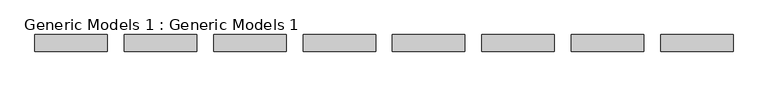
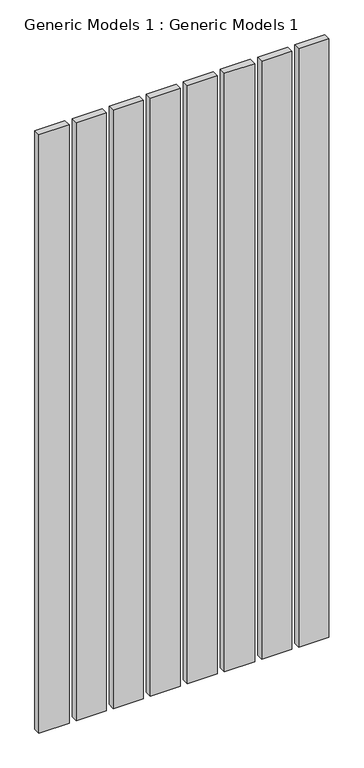
"""IFC4 building model written with IfcOpenShell, lengths in millimetres: proxy geometry, Generic Models 1 : Generic Models 1."""

from ifc_helpers import new_model, si_unit, origin, origin_with_axes, place, context, project, spatial, polyline, outline, extrude, source, transform, mapped, element, save


def generic_models_1_generic_models_1_37e6f81f(model_context):
    return source(origin(), model_context, "Body", "SweptSolid", [
        extrude(outline(polyline([(-12021.880705, -5332.9027976), (-11913.168705, -5332.9027976), (-11913.168705, -5358.3027976), (-12021.880705, -5358.3027976), (-12021.880705, -5332.9027976)])), origin_with_axes(), (0.0, 0.0, 1.0), 2286.0),
        extrude(outline(polyline([(-12155.992705, -5332.9027976), (-12047.280705, -5332.9027976), (-12047.280705, -5358.3027976), (-12155.992705, -5358.3027976), (-12155.992705, -5332.9027976)])), origin_with_axes(), (0.0, 0.0, 1.0), 2286.0),
        extrude(outline(polyline([(-12290.104705, -5332.9027976), (-12181.392705, -5332.9027976), (-12181.392705, -5358.3027976), (-12290.104705, -5358.3027976), (-12290.104705, -5332.9027976)])), origin_with_axes(), (0.0, 0.0, 1.0), 2286.0),
        extrude(outline(polyline([(-12424.216705, -5332.9027976), (-12315.504705, -5332.9027976), (-12315.504705, -5358.3027976), (-12424.216705, -5358.3027976), (-12424.216705, -5332.9027976)])), origin_with_axes(), (0.0, 0.0, 1.0), 2286.0),
        extrude(outline(polyline([(-12558.328705, -5332.9027976), (-12449.616705, -5332.9027976), (-12449.616705, -5358.3027976), (-12558.328705, -5358.3027976), (-12558.328705, -5332.9027976)])), origin_with_axes(), (0.0, 0.0, 1.0), 2286.0),
        extrude(outline(polyline([(-12692.440705, -5332.9027976), (-12583.728705, -5332.9027976), (-12583.728705, -5358.3027976), (-12692.440705, -5358.3027976), (-12692.440705, -5332.9027976)])), origin_with_axes(), (0.0, 0.0, 1.0), 2286.0),
        extrude(outline(polyline([(-12826.552705, -5332.9027976), (-12717.840705, -5332.9027976), (-12717.840705, -5358.3027976), (-12826.552705, -5358.3027976), (-12826.552705, -5332.9027976)])), origin_with_axes(), (0.0, 0.0, 1.0), 2286.0),
        extrude(outline(polyline([(-12960.664705, -5332.9027976), (-12851.952705, -5332.9027976), (-12851.952705, -5358.3027976), (-12960.664705, -5358.3027976), (-12960.664705, -5332.9027976)])), origin_with_axes(), (0.0, 0.0, 1.0), 2286.0),
    ])


if __name__ == "__main__":
    model = new_model("IFC4")
    model_context = context("Model", 3, world=origin())
    ifc_project = project(units=[si_unit("LENGTHUNIT", "METRE", prefix="MILLI")], contexts=[model_context])
    site = spatial("IfcSite", under=ifc_project)
    building = spatial("IfcBuilding", under=site)
    placement = place(None, origin())
    generic_models_1_generic_models_1_shape = generic_models_1_generic_models_1_37e6f81f(model_context)
    element("IfcBuildingElementProxy", 1, Name="Generic Models 1 : Generic Models 1", ObjectType="Generic Models 1 : Generic Models 1", at=placement, inside=building, context=model_context, shape_type="MappedRepresentation", body=[
        mapped(generic_models_1_generic_models_1_shape, transform((0.0, 0.0, 0.0), x_axis=(1.0, 0.0, 0.0), y_axis=(0.0, 1.0, 0.0), z_axis=(0.0, 0.0, 1.0))),
    ])
    save(model, "model.ifc")

# Revit data of these elements
# Element 1 (IfcBuildingElementProxy, "Generic Models 1 : Generic Models 1")
#   Materials on its faces: "Wood Planks"
# Materials
#   "Wood Planks": class "Wood", colour RGB 129 72 39, transparency 0, Description = "Physical material.", Cost = 0
